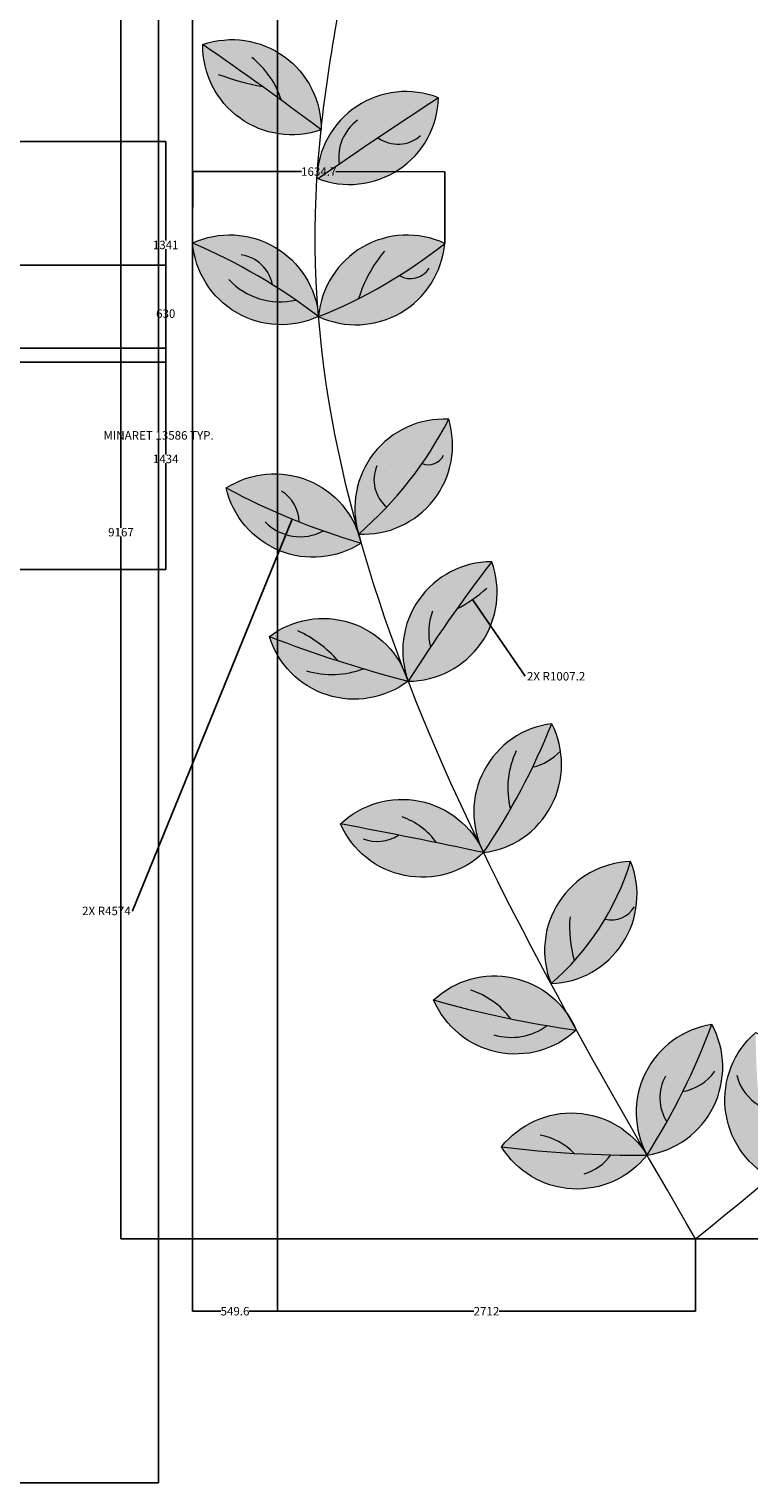
# Model space of a CAD drawing. Units: millimetres. Extents: x 8570 to 49085, y 3782 to 24863.
# Tile 12 of 15: x 35169 to 39837, y 5902 to 15329. Entities that reach past the tile are written whole.
import ezdxf

# ---------------------------------------------------------------- set-up
doc = ezdxf.new("R2010")
doc.units = ezdxf.units.MM
doc.header["$MEASUREMENT"] = 0
doc.header["$PDMODE"] = 3
for name, color, linetype, lineweight in [('A-ANNO-DIMS', 2, 'Continuous', 18), ('A-DETL-FOLI', 7, 'Continuous', 13), ('A-DETL-PATT', 3, 'Continuous', 13), ('A-DETL-STEM', 28, 'Continuous', 18)]:
    doc.layers.add(name, color=color, linetype=linetype, lineweight=lineweight)
doc.styles.get("Standard").update_dxf_attribs({"font": 'arial.ttf'})
doc.dimstyles.get("Standard").update_dxf_attribs({"dimtxt": 55, "dimasz": 0.18, "dimexe": 0.18, "dimexo": 0.0625, "dimgap": 0.09, "dimtad": 0, "dimtih": 1, "dimtoh": 1, "dimdec": 0, "dimzin": 0, "dimdsep": 46, "dimtxsty": 'Standard', "dimcen": 0.09, "dimadec": 0, "dimazin": 0, "dimtfac": 1, "dimtdec": 0, "dimtofl": 0, "dimtmove": 0, "dimatfit": 3, "dimfxl": 1, "dimtolj": 1, "dimtzin": 0, "dimarcsym": 0})

# ---------------------------------------------------------------- blocks, each defined once
blk = doc.blocks.new('*D15')
at = {"layer": 'A-ANNO-DIMS', "color": 0, "lineweight": -2, "transparency": 16777216}
for p, q in [((33971.1, 19487.3), (36009.1, 19487.3)), ((36008.9, 19487.1), (36008.9, 12722.6)), ((36008.9, 5901.7), (36008.9, 12666.2)), ((33971.1, 5901.5), (36009.1, 5901.5))]:
    blk.add_line(p, q, dxfattribs=at)
at = {"layer": 'A-ANNO-DIMS', "color": 0, "transparency": 16777216}
for points in [[(36008.8, 19487.1), (36008.9, 19487.1), (36008.9, 19487.3)], [(36008.8, 5901.7), (36008.9, 5901.7), (36008.9, 5901.5)]]:
    blk.add_solid(points, dxfattribs=at)
at = {"layer": 'Defpoints', "color": 0, "transparency": 16777216}
for p in [(33971, 19487.3), (36008.9, 19487.3), (33971, 5901.5)]:
    blk.add_point(p, dxfattribs=at)
at = {"layer": 'A-ANNO-DIMS', "color": 0, "transparency": 16777216, "insert": (36008.9, 12694.4), "char_height": 55, "attachment_point": 5}
blk.add_mtext('\\A1;MINARET 13586 TYP.', dxfattribs=at)
blk = doc.blocks.new('*D50')
at = {"layer": 'A-ANNO-DIMS', "color": 0, "lineweight": -2, "transparency": 16777216}
for p, q in [((22407.6, 13259), (36055.2, 13259)), ((36055, 13258.8), (36055, 12570.2)), ((36055, 11825.2), (36055, 12513.8)), ((24254.1, 11825), (36055.2, 11825))]:
    blk.add_line(p, q, dxfattribs=at)
at = {"layer": 'A-ANNO-DIMS', "color": 0, "transparency": 16777216}
for points in [[(36055, 13258.8), (36055, 13258.8), (36055, 13259)], [(36055, 11825.2), (36055, 11825.2), (36055, 11825)]]:
    blk.add_solid(points, dxfattribs=at)
at = {"layer": 'Defpoints', "color": 0, "transparency": 16777216}
for p in [(22407.5, 13259), (36055, 13259), (24254, 11825)]:
    blk.add_point(p, dxfattribs=at)
at = {"layer": 'A-ANNO-DIMS', "color": 0, "transparency": 16777216, "insert": (36055, 12542), "char_height": 55, "attachment_point": 5}
blk.add_mtext('\\A1;1434', dxfattribs=at)
blk = doc.blocks.new('*D51')
at = {"layer": 'A-ANNO-DIMS', "color": 0, "lineweight": -2, "transparency": 16777216}
for p, q in [((25004.1, 14600), (36055.2, 14600)), ((36055, 14599.8), (36055, 13957.7)), ((36055, 13259.2), (36055, 13901.3)), ((22407.6, 13259), (36055.2, 13259))]:
    blk.add_line(p, q, dxfattribs=at)
at = {"layer": 'A-ANNO-DIMS', "color": 0, "transparency": 16777216}
for points in [[(36055, 14599.8), (36055, 14599.8), (36055, 14600)], [(36055, 13259.2), (36055, 13259.2), (36055, 13259)]]:
    blk.add_solid(points, dxfattribs=at)
at = {"layer": 'Defpoints', "color": 0, "transparency": 16777216}
for p in [(25004, 14600), (36055, 14600), (22407.5, 13259)]:
    blk.add_point(p, dxfattribs=at)
at = {"layer": 'A-ANNO-DIMS', "color": 0, "transparency": 16777216, "insert": (36055, 13929.5), "char_height": 55, "attachment_point": 5}
blk.add_mtext('\\A1;1341', dxfattribs=at)
blk = doc.blocks.new('*D68')
at = {"layer": 'A-ANNO-DIMS', "color": 0, "lineweight": -2, "transparency": 16777216}
for p, q in [((29204.1, 13799), (36055.2, 13799)), ((36055, 13798.8), (36055, 13512.2)), ((36055, 13169.2), (36055, 13455.8)), ((28954.1, 13169), (36055.2, 13169))]:
    blk.add_line(p, q, dxfattribs=at)
at = {"layer": 'A-ANNO-DIMS', "color": 0, "transparency": 16777216}
for points in [[(36055, 13798.8), (36055, 13798.8), (36055, 13799)], [(36055, 13169.2), (36055, 13169.2), (36055, 13169)]]:
    blk.add_solid(points, dxfattribs=at)
at = {"layer": 'Defpoints', "color": 0, "transparency": 16777216}
for p in [(29204, 13799), (36055, 13799), (28954, 13169)]:
    blk.add_point(p, dxfattribs=at)
at = {"layer": 'A-ANNO-DIMS', "color": 0, "transparency": 16777216, "insert": (36055, 13484), "char_height": 55, "attachment_point": 5}
blk.add_mtext('\\A1;630', dxfattribs=at)
blk = doc.blocks.new('*D72')
at = {"layer": 'A-ANNO-DIMS', "color": 0, "lineweight": -2, "transparency": 16777216}
for p, q in [((36229.4, 13941.8), (36229.4, 17114.8)), ((36229.6, 17114.6), (40660.1, 17114.6)), ((45255, 17114.6), (40824.5, 17114.6)), ((45255.2, 15109.6), (45255.2, 17114.8))]:
    blk.add_line(p, q, dxfattribs=at)
at = {"layer": 'A-ANNO-DIMS', "color": 0, "transparency": 16777216}
for points in [[(36229.6, 17114.7), (36229.6, 17114.6), (36229.4, 17114.6)], [(45255, 17114.7), (45255, 17114.6), (45255.2, 17114.6)]]:
    blk.add_solid(points, dxfattribs=at)
at = {"layer": 'Defpoints', "color": 0, "transparency": 16777216}
for p in [(45255.2, 17114.6), (45255.2, 15109.5), (36229.4, 13941.8)]:
    blk.add_point(p, dxfattribs=at)
at = {"layer": 'A-ANNO-DIMS', "color": 0, "transparency": 16777216, "insert": (40742.3, 17114.6), "char_height": 55, "attachment_point": 5}
blk.add_mtext('\\A1;9026', dxfattribs=at)
blk = doc.blocks.new('*D73')
at = {"layer": 'A-ANNO-DIMS', "color": 0, "lineweight": -2, "transparency": 16777216}
for p, q in [((36779, 16650.1), (35764.8, 16650.1)), ((35764.9, 16649.9), (35764.9, 12095)), ((35764.9, 7483.7), (35764.9, 12038.6)), ((39490.9, 7483.5), (35764.8, 7483.5))]:
    blk.add_line(p, q, dxfattribs=at)
at = {"layer": 'A-ANNO-DIMS', "color": 0, "transparency": 16777216}
for points in [[(35764.9, 16649.9), (35765, 16649.9), (35764.9, 16650.1)], [(35764.9, 7483.7), (35765, 7483.7), (35764.9, 7483.5)]]:
    blk.add_solid(points, dxfattribs=at)
at = {"layer": 'Defpoints', "color": 0, "transparency": 16777216}
for p in [(35764.9, 16650.1), (36779.1, 16650.1), (39491, 7483.5)]:
    blk.add_point(p, dxfattribs=at)
at = {"layer": 'A-ANNO-DIMS', "color": 0, "transparency": 16777216, "insert": (35764.9, 12066.8), "char_height": 55, "attachment_point": 5}
blk.add_mtext('\\A1;9167', dxfattribs=at)
blk = doc.blocks.new('*D74')
at = {"layer": 'A-ANNO-DIMS', "color": 0, "lineweight": -2, "transparency": 16777216}
for p, q in [((36779.1, 16650.1), (36779.1, 7015)), ((36229.4, 13941.7), (36229.4, 7015)), ((36229.6, 7015.1), (36411.4, 7015.1)), ((36778.9, 7015.1), (36597.1, 7015.1))]:
    blk.add_line(p, q, dxfattribs=at)
at = {"layer": 'A-ANNO-DIMS', "color": 0, "transparency": 16777216}
for points in [[(36229.6, 7015.2), (36229.6, 7015.1), (36229.4, 7015.1)], [(36778.9, 7015.2), (36778.9, 7015.1), (36779.1, 7015.1)]]:
    blk.add_solid(points, dxfattribs=at)
at = {"layer": 'Defpoints', "color": 0, "transparency": 16777216}
for p in [(36779.1, 16650.1), (36229.4, 13941.8), (36779.1, 7015.1)]:
    blk.add_point(p, dxfattribs=at)
at = {"layer": 'A-ANNO-DIMS', "color": 0, "transparency": 16777216, "insert": (36504.3, 7015.1), "char_height": 55, "attachment_point": 5}
blk.add_mtext('\\A1;549.6', dxfattribs=at)
blk = doc.blocks.new('*D75')
at = {"layer": 'A-ANNO-DIMS', "color": 0, "lineweight": -2, "transparency": 16777216}
for p, q in [((36779.1, 16650.1), (36779.1, 7015)), ((39491, 7483.4), (39491, 7015)), ((36779.2, 7015.1), (38052.6, 7015.1)), ((39490.8, 7015.1), (38217.4, 7015.1))]:
    blk.add_line(p, q, dxfattribs=at)
at = {"layer": 'A-ANNO-DIMS', "color": 0, "transparency": 16777216}
for points in [[(36779.2, 7015.2), (36779.2, 7015.1), (36779.1, 7015.1)], [(39490.8, 7015.2), (39490.8, 7015.1), (39491, 7015.1)]]:
    blk.add_solid(points, dxfattribs=at)
at = {"layer": 'Defpoints', "color": 0, "transparency": 16777216}
for p in [(36779.1, 16650.1), (39491, 7483.5), (39491, 7015.1)]:
    blk.add_point(p, dxfattribs=at)
at = {"layer": 'A-ANNO-DIMS', "color": 0, "transparency": 16777216, "insert": (38135, 7015.1), "char_height": 55, "attachment_point": 5}
blk.add_mtext('\\A1;2712', dxfattribs=at)
blk = doc.blocks.new('*D76')
at = {"layer": 'A-ANNO-DIMS', "color": 0, "lineweight": -2, "transparency": 16777216}
for p, q in [((45255.3, 15109.5), (45721.9, 15109.5)), ((45721.7, 15109.3), (45721.7, 11324.7)), ((45721.7, 7483.7), (45721.7, 11268.3)), ((39491.1, 7483.5), (45721.9, 7483.5))]:
    blk.add_line(p, q, dxfattribs=at)
at = {"layer": 'A-ANNO-DIMS', "color": 0, "transparency": 16777216}
for points in [[(45721.6, 15109.3), (45721.7, 15109.3), (45721.7, 15109.5)], [(45721.6, 7483.7), (45721.7, 7483.7), (45721.7, 7483.5)]]:
    blk.add_solid(points, dxfattribs=at)
at = {"layer": 'Defpoints', "color": 0, "transparency": 16777216}
for p in [(45255.2, 15109.5), (45721.7, 15109.5), (39491, 7483.5)]:
    blk.add_point(p, dxfattribs=at)
at = {"layer": 'A-ANNO-DIMS', "color": 0, "transparency": 16777216, "insert": (45721.7, 11296.5), "char_height": 55, "attachment_point": 5}
blk.add_mtext('\\A1;7626', dxfattribs=at)
blk = doc.blocks.new('*D78')
at = {"layer": 'A-ANNO-DIMS', "color": 0, "lineweight": -2, "transparency": 16777216}
for p, q in [((36229.4, 13941.8), (36230, 14406.4)), ((36230.2, 14406.3), (36935.7, 14405.4)), ((37864.5, 14404.2), (37159, 14405.1)), ((37864.1, 13939.7), (37864.7, 14404.3))]:
    blk.add_line(p, q, dxfattribs=at)
at = {"layer": 'A-ANNO-DIMS', "color": 0, "transparency": 16777216}
for points in [[(36230.2, 14406.3), (36230.2, 14406.2), (36230, 14406.3)], [(37864.5, 14404.2), (37864.5, 14404.1), (37864.7, 14404.2)]]:
    blk.add_solid(points, dxfattribs=at)
at = {"layer": 'Defpoints', "color": 0, "transparency": 16777216}
for p in [(37864.7, 14404.2), (36229.4, 13941.8), (37864.1, 13939.7)]:
    blk.add_point(p, dxfattribs=at)
at = {"layer": 'A-ANNO-DIMS', "color": 0, "transparency": 16777216, "insert": (37047.4, 14405.2), "char_height": 55, "attachment_point": 5}
blk.add_mtext('\\A1;1634.7', dxfattribs=at)
blk = doc.blocks.new('*D95')
at = {"layer": 'A-ANNO-DIMS', "color": 0, "lineweight": -2, "transparency": 16777216}
for p, q in [((48826.8, 12322.2), (42401, 10673.8)), ((31690.9, 7926.2), (31691.1, 7926.2)), ((31691, 7926.2), (31691, 7926.3))]:
    blk.add_line(p, q, dxfattribs=at)
at = {"layer": 'A-ANNO-DIMS', "color": 0, "transparency": 16777216}
blk.add_solid([(42401, 10673.8), (42401, 10673.7), (42400.9, 10673.7)], dxfattribs=at)
at = {"layer": 'Defpoints', "color": 0, "transparency": 16777216}
for p in [(42400.9, 10673.7), (31691, 7926.2)]:
    blk.add_point(p, dxfattribs=at)
at = {"layer": 'A-ANNO-DIMS', "color": 0, "transparency": 16777216, "insert": (48956.7, 12322.2), "char_height": 55, "attachment_point": 5}
blk.add_mtext('\\A1;R11057', dxfattribs=at)
blk = doc.blocks.new('*D97')
at = {"layer": 'A-ANNO-DIMS', "color": 0, "lineweight": -2, "transparency": 16777216}
for p, q in [((38605.2, 16386.9), (38605.4, 16386.9)), ((38605.3, 16386.8), (38605.3, 16387)), ((35838.6, 9611), (36876, 12151.8)), ((35838.4, 9611), (35838.6, 9611))]:
    blk.add_line(p, q, dxfattribs=at)
at = {"layer": 'A-ANNO-DIMS', "color": 0, "transparency": 16777216}
blk.add_solid([(36876, 12151.8), (36876.1, 12151.8), (36876.1, 12152)], dxfattribs=at)
at = {"layer": 'Defpoints', "color": 0, "transparency": 16777216}
for p in [(38605.3, 16386.9), (36876.1, 12152)]:
    blk.add_point(p, dxfattribs=at)
at = {"layer": 'A-ANNO-DIMS', "color": 0, "transparency": 16777216, "insert": (35670.4, 9611), "char_height": 55, "attachment_point": 5}
blk.add_mtext('\\A1;2X R4574', dxfattribs=at)
blk = doc.blocks.new('*D99')
at = {"layer": 'A-ANNO-DIMS', "color": 0, "lineweight": -2, "transparency": 16777216}
for p, q in [((37473.5, 12460.3), (37473.6, 12460.3)), ((37473.6, 12460.2), (37473.6, 12460.4)), ((38386.6, 11132.5), (38044.3, 11630.3)), ((38386.8, 11132.5), (38386.6, 11132.5))]:
    blk.add_line(p, q, dxfattribs=at)
at = {"layer": 'A-ANNO-DIMS', "color": 0, "transparency": 16777216}
blk.add_solid([(38044.3, 11630.3), (38044.3, 11630.2), (38044.2, 11630.4)], dxfattribs=at)
at = {"layer": 'Defpoints', "color": 0, "transparency": 16777216}
for p in [(37473.6, 12460.3), (38044.2, 11630.4)]:
    blk.add_point(p, dxfattribs=at)
at = {"layer": 'A-ANNO-DIMS', "color": 0, "transparency": 16777216, "insert": (38586.6, 11132.5), "char_height": 55, "attachment_point": 5}
blk.add_mtext('\\A1;2X R1007.2', dxfattribs=at)

msp = doc.modelspace()

# ---------------------------------------------------------------- hatches: boundary and pattern name
at = {"layer": 'A-DETL-PATT'}
h = msp.add_hatch(color=256, dxfattribs=at)
h.dxf.hatch_style = 1
h.paths.add_polyline_path([(36295.31, 15228.7, 0.5205671), (37062.67, 14676.08, 0.0103411)])
h = msp.add_hatch(color=256, dxfattribs=at)
h.dxf.hatch_style = 1
h.paths.add_polyline_path([(36295.31, 15228.7, -0.0103411), (37062.67, 14676.08, 0.5205671)])
h = msp.add_hatch(color=256, dxfattribs=at)
h.dxf.hatch_style = 1
h.paths.add_polyline_path([(37823.87, 14883.96, 0.5205671), (37035.68, 14361.49, 0.0037395), (37043.74, 14358.39, -0.0070598)])
h = msp.add_hatch(color=256, dxfattribs=at)
h.dxf.hatch_style = 1
h.paths.add_polyline_path([(37823.87, 14883.96, 0.0070598), (37043.74, 14358.39, 0.5158234)])
h = msp.add_hatch(color=256, dxfattribs=at)
h.dxf.hatch_style = 1
h.paths.add_polyline_path([(36229.45, 13941.76, -0.520567), (37046.17, 13465.11, -0.520567), (37864.11, 13939.66, -0.520567), (37046.17, 13465.11, -0.520567)])
h = msp.add_hatch(color=256, dxfattribs=at)
h.dxf.hatch_style = 1
h.paths.add_polyline_path([(36229.45, 13941.76, -0.0616433), (37046.17, 13465.11, 0.5205671)])
h = msp.add_hatch(color=256, dxfattribs=at)
h.dxf.hatch_style = 1
h.paths.add_polyline_path([(37864.11, 13939.66, 0.5205671), (37046.17, 13465.11, 0.0744626)], flags=17)
h = msp.add_hatch(color=256, dxfattribs=at)
h.dxf.hatch_style = 1
h.paths.add_polyline_path([(36229.45, 13941.76, 0.520567), (37046.17, 13465.11, 0.0616433)], flags=17)
h = msp.add_hatch(color=256, dxfattribs=at)
h.dxf.hatch_style = 1
edge = h.paths.add_edge_path()
edge.add_arc((37858.74, 12222.44), 577.2, 86.889324, 194.195037)
edge.add_spline(control_points=[(37299.16, 12080.9), (37301.57, 12072.18), (37304, 12063.46), (37306.43, 12054.75)], knot_values=[4911.3561457, 4911.3561457, 4911.3561457, 4911.3561457, 4938.9064516, 4938.9064516, 4938.9064516, 4938.9064516], degree=3, periodic=0)
edge.add_arc((35669.24, 13939.89), 2496.83, 310.973454, 332.805194)
h = msp.add_hatch(color=256, dxfattribs=at)
h.dxf.hatch_style = 1
h.paths.add_polyline_path([(37890.06, 12798.79, -0.0955481), (37306.43, 12054.75, 0.5205671)])
h = msp.add_hatch(color=256, dxfattribs=at)
h.dxf.hatch_style = 1
h.paths.add_polyline_path([(36447.63, 12353.41, 0.0518202), (37323.1, 11995.94, 0.520567)])
h = msp.add_hatch(color=256, dxfattribs=at)
h.dxf.hatch_style = 1
h.paths.add_polyline_path([(36447.63, 12353.41, 0.5205671), (37323.1, 11995.94, -0.0518202)])
h = msp.add_hatch(color=256, dxfattribs=at)
h.dxf.hatch_style = 1
h.paths.add_polyline_path([(38169.31, 11875.19, 0.5048203), (37617.86, 11127.77, -0.0124698), (37627.03, 11100.49, -0.0213914)])
h = msp.add_hatch(color=256, dxfattribs=at)
h.dxf.hatch_style = 1
h.paths.add_polyline_path([(38169.31, 11875.19, 0.0213914), (37627.03, 11100.49, 0.5205671)])
h = msp.add_hatch(color=256, dxfattribs=at)
h.dxf.hatch_style = 1
h.paths.add_polyline_path([(36726.91, 11390.34, 0.0289339), (37627.03, 11100.49, -0.0124698), (37617.86, 11127.77, 0.5048203)])
h = msp.add_hatch(color=256, dxfattribs=at)
h.dxf.hatch_style = 1
h.paths.add_polyline_path([(37627.03, 11100.49, -0.0289339), (36726.91, 11390.34, 0.5205671)])
h = msp.add_hatch(color=256, dxfattribs=at)
h.dxf.hatch_style = 1
h.paths.add_polyline_path([(38558.32, 10824.89, 0.5013788), (38101.47, 10020.52, -0.0152167), (38116.54, 9988.79, 0.0525775)])
h = msp.add_hatch(color=256, dxfattribs=at)
h.dxf.hatch_style = 1
h.paths.add_polyline_path([(38558.32, 10824.89, -0.0171383), (38433.65, 10542.15, 0.1348282), (38615.59, 10646.7, 0.0816048)])
h = msp.add_hatch(color=256, dxfattribs=at)
h.dxf.hatch_style = 1
h.paths.add_polyline_path([(38615.59, 10646.7, -0.1348282), (38433.65, 10542.15, -0.0354074), (38116.54, 9988.79, 0.4210746)])
h = msp.add_hatch(color=256, dxfattribs=at)
h.dxf.hatch_style = 1
h.paths.add_polyline_path([(37189.36, 10174.71, -0.0070162), (38116.54, 9988.79, -0.0152167), (38101.47, 10020.52, 0.5013788)])
h = msp.add_hatch(color=256, dxfattribs=at)
h.dxf.hatch_style = 1
h.paths.add_polyline_path([(37189.36, 10174.71, 0.5205671), (38116.54, 9988.79, 0.0070162)])
h = msp.add_hatch(color=256, dxfattribs=at)
h.dxf.hatch_style = 1
h.paths.add_polyline_path([(39069.9, 9931.39, 0.520567), (38553.65, 9139.1, 0.1409243)])
h = msp.add_hatch(color=256, dxfattribs=at)
h.dxf.hatch_style = 1
h.paths.add_polyline_path([(39069.9, 9931.39, -0.1409243), (38553.65, 9139.1, 0.5205671)])
h = msp.add_hatch(color=256, dxfattribs=at)
h.dxf.hatch_style = 1
edge = h.paths.add_edge_path()
edge.add_spline(control_points=[(38717.84, 8838.28), (38699.24, 8871.96), (38680.7, 8905.65), (38662.23, 8939.34)], knot_values=[1468.6434181, 1468.6434181, 1468.6434181, 1468.6434181, 1577.9808208, 1577.9808208, 1577.9808208, 1577.9808208], degree=3, periodic=0)
edge.add_arc((38186.86, 8611.95), 577.2, 34.555708, 133.086732)
edge.add_arc((39646, 15528.1), 6753.9, 254.072359, 262.101105)
h = msp.add_hatch(color=256, dxfattribs=at)
h.dxf.hatch_style = 1
h.paths.add_polyline_path([(37792.57, 9033.49, 0.5205671), (38717.84, 8838.28, -0.0350464)])
h = msp.add_hatch(color=256, dxfattribs=at)
h.dxf.hatch_style = 1
h.paths.add_polyline_path([(39596.97, 8874.13, 0.520567), (39176.6, 8027.06, 0.0505737)])
h = msp.add_hatch(color=256, dxfattribs=at)
h.dxf.hatch_style = 1
h.paths.add_polyline_path([(39596.97, 8874.13, -0.0505737), (39176.6, 8027.06, 0.5205671)])
h = msp.add_hatch(color=256, dxfattribs=at)
h.dxf.hatch_style = 1
h.paths.add_polyline_path([(39881.17, 8822.47, 0.5205671), (39976.57, 7881.66, -0.0505737)])
h = msp.add_hatch(color=256, dxfattribs=at)
h.dxf.hatch_style = 1
h.paths.add_polyline_path([(38232.5, 8081.06, 0.0328597), (39176.6, 8027.06, 0.5205671)])
h = msp.add_hatch(color=256, dxfattribs=at)
h.dxf.hatch_style = 1
h.paths.add_polyline_path([(38232.5, 8081.06, 0.520567), (39176.6, 8027.06, -0.0328597)])

# ---------------------------------------------------------------- linework, layer by layer
at = {"layer": 'A-DETL-FOLI'}
for points in [[(37062.67, 14676.08, -0.520567), (36295.31, 15228.7, -0.520567)], [(37035.68, 14361.49, 0.5205671), (37823.87, 14883.96, 0.5205671)], [(37046.17, 13465.11, -0.5205671), (36229.45, 13941.76, -0.5205671)], [(37046.17, 13465.11, 0.5205671), (37864.11, 13939.66, 0.5205671)], [(37306.43, 12054.75, 0.5205671), (37890.06, 12798.79, 0.5205671)], [(37323.1, 11995.94, -0.5205671), (36447.63, 12353.41, -0.5205671)], [(37627.03, 11100.49, 0.5205671), (38169.31, 11875.19, 0.5205671)], [(37627.03, 11100.49, -0.5205671), (36726.91, 11390.34, -0.5205671)], [(38116.54, 9988.79, 0.5205671), (38558.32, 10824.89, 0.5205671)], [(38116.54, 9988.79, -0.5205671), (37189.36, 10174.71, -0.5205671)], [(38553.65, 9139.1, 0.5205671), (39069.9, 9931.39, 0.5205671)], [(38717.84, 8838.28, -0.5205671), (37792.57, 9033.49, -0.5205671)], [(39176.6, 8027.06, 0.5205671), (39596.97, 8874.13, 0.5205671)], [(39976.57, 7881.66, -0.5205671), (39881.17, 8822.47, -0.5205671)], [(39176.6, 8027.06, -0.5205671), (38232.5, 8081.06, -0.5205671)]]:
    msp.add_lwpolyline(points, format="xyb", close=True, dxfattribs=at)
for centre, radius, start, end in [((23320.55, -3596.85), 22863.63, 53.055085, 55.425), ((36271.19, 14703.58), 558.08, 17.051895, 52.17229), ((37032.61, 16773.69), 1850.87, 249.886877, 259.075602), ((56044.44, -13003.46), 33312.13, 123.15906, 124.777015), ((37476.65, 14496.91), 299.94, 126.268669, 188.510463), ((37560.28, 14802.57), 219.96, 234.307882, 311.816375), ((34712.07, 10403.74), 3849.69, 52.676825, 66.786584), ((36509.64, 13624.91), 242.64, 10.975798, 81.833743), ((35870.73, 16433.32), 3192.47, 291.604155, 308.638293), ((38138.63, 13327.54), 870.37, 139.909154, 163.015855), ((37643.87, 13851.05), 139.85, 238.748189, 328.478767), ((36798.02, 14020.4), 460, 223.326558, 282.722995), ((35669.24, 13939.89), 2496.83, 310.973454, 332.805194), ((37757.22, 12612.81), 108.88, 248.41912, 334.400323), ((37634.06, 12406.03), 228.57, 156.595932, 230.447825), ((38605.31, 16386.92), 4574.36, 241.855973, 253.721673), ((36680, 12126.54), 240.93, 1.777734, 58.42246), ((36927.75, 12356.22), 318.74, 224.316548, 298.113447), ((46947.91, 5153.12), 11056.67, 142.557509, 147.459302), ((37473.56, 12460.31), 1007.16, 297.810827, 311.215558), ((38161.62, 11414.85), 401.41, 159.701903, 193.541189), ((36563.49, 10690.41), 815.46, 41.653998, 64.77332), ((39679.3, 19016.27), 8177.5, 248.836039, 255.465354), ((37132.6, 11733.77), 589.63, 253.685845, 290.393138), ((34372.89, 12501.66), 4508.82, 326.129117, 338.167916), ((38838.71, 10406.9), 565.03, 154.67912, 194.042291), ((38334.29, 10925.66), 396.17, 284.524319, 315.239446), ((37434.91, 9784.63), 462.08, 35.512434, 70.735424), ((31028.6, -22953.94), 33696.62, 77.857396, 79.465354), ((37425.74, 10310.28), 249.31, 248.564819, 303.69009), ((37434.17, 10432.88), 1710.88, 310.86914, 342.95532), ((38947.21, 9723.28), 170.45, 255.51577, 329.955221), ((39431.86, 9504.6), 758.17, 174.789648, 196.615742), ((37864.29, 8585.96), 538.45, 37.132204, 71.607072), ((39646, 15528.1), 6753.9, 254.072359, 262.101105), ((38297.06, 9180.64), 390.09, 252.908213, 306.526234), ((35210.23, 10523.3), 4686.5, 327.815771, 339.396549), ((39546.84, 8398.85), 287.73, 150.652053, 212.713005), ((39357.43, 8748.48), 312.66, 279.345292, 325.49765), ((40061.17, 8620.56), 312.66, 193.8989, 240.051258), ((38402.78, 7743.64), 421.31, 44.425388, 79.130728), ((39114.91, 15229.08), 7202.28, 262.962572, 270.490744), ((38675.82, 8218.4), 326.41, 286.427156, 324.507445)]:
    msp.add_arc(centre, radius, start, end, dxfattribs=at)
at = {"layer": 'A-DETL-STEM'}
for points in [[(39491, 7483.5), (38190.27, 9726.55), (36625.55, 12424.85), (37154.41, 15335.42), (37243.63, 15826.48)], [(39491, 7483.5), (41497.86, 9125.36), (43912.02, 11100.44), (44441.22, 14010.96), (44530.5, 14502)]]:
    msp.add_open_spline(points, degree=3, knots=[0, 0, 0, 0, 7301.1442939, 8782.9420196, 8782.9420196, 8782.9420196, 8782.9420196], dxfattribs=at)

# ---------------------------------------------------------------- dimensions: what is measured, and where the dimension line sits
at = {"layer": 'A-ANNO-DIMS'}
dim = msp.add_linear_dim(base=(36008.87, 19487.32), p1=(33971, 5901.5), p2=(33971, 19487.32), angle=90, text='MINARET <> TYP.', dimstyle='Standard', override={"dimdec": 0, "dimlfac": 1, "dimrnd": 0, "dimzin": 0, "dimdsep": 46, "dimlunit": 2}, dxfattribs=at)
dim.commit()
dim.dimension.update_dxf_attribs({"geometry": '*D15', "text_midpoint": (36008.87, 12694.41)})
for base, p1, p2, override, picture, middle in [((45255.2, 17114.63), (36229.45, 13941.76), (45255.2, 15109.49), {"dimdec": 0, "dimlfac": 1, "dimrnd": 0, "dimzin": 0, "dimdsep": 46, "dimlunit": 2}, '*D72', (40742.32, 17114.63)), ((36779.06, 7015.15), (36229.45, 13941.76), (36779.06, 16650.13), {"dimdec": 1, "dimlfac": 1, "dimrnd": 0, "dimzin": 0, "dimdsep": 46, "dimlunit": 2}, '*D74', (36504.25, 7015.15)), ((39491, 7015.15), (36779.06, 16650.13), (39491, 7483.5), {"dimdec": 0, "dimlfac": 1, "dimrnd": 0, "dimzin": 0, "dimdsep": 46, "dimlunit": 2}, '*D75', (38135.03, 7015.15))]:
    dim = msp.add_linear_dim(base=base, p1=p1, p2=p2, dimstyle='Standard', override=override, dxfattribs=at)
    dim.commit()
    dim.dimension.update_dxf_attribs({"geometry": picture, "text_midpoint": middle})
for base, p1, p2, angle, override, picture, middle in [((35764.95, 16650.13), (39491, 7483.5), (36779.06, 16650.13), 90, {"dimdec": 0, "dimlfac": 1, "dimrnd": 0, "dimzin": 0, "dimdsep": 46, "dimlunit": 2}, '*D73', (35764.95, 12066.81)), ((45721.68, 15109.49), (39491, 7483.5), (45255.2, 15109.49), 90, {"dimdec": 0, "dimlfac": 1, "dimrnd": 0, "dimzin": 0, "dimdsep": 46, "dimlunit": 2}, '*D76', (45721.68, 11296.49)), ((36055, 14600), (22407.5, 13259), (25004, 14600), 90, {"dimdec": 0, "dimlfac": 1, "dimrnd": 0, "dimzin": 0, "dimdsep": 46, "dimlunit": 2}, '*D51', (36055, 13929.5)), ((37864.71, 14404.16), (36229.45, 13941.76), (37864.11, 13939.66), 359.926464, {"dimdec": 1, "dimlfac": 1, "dimrnd": 0, "dimzin": 0, "dimdsep": 46, "dimlunit": 2}, '*D78', (37047.38, 14405.21)), ((36055, 13799), (28954, 13169), (29204, 13799), 90, {"dimdec": 0, "dimlfac": 1, "dimrnd": 0, "dimzin": 0, "dimdsep": 46, "dimlunit": 2}, '*D68', (36055, 13484)), ((36055, 13259), (24254, 11825), (22407.5, 13259), 90, {"dimdec": 0, "dimlfac": 1, "dimrnd": 0, "dimzin": 0, "dimdsep": 46, "dimlunit": 2}, '*D50', (36055, 12542))]:
    dim = msp.add_linear_dim(base=base, p1=p1, p2=p2, angle=angle, dimstyle='Standard', override=override, dxfattribs=at)
    dim.commit()
    dim.dimension.update_dxf_attribs({"geometry": picture, "text_midpoint": middle})
for center, mpoint, override, picture, middle in [((38605.31, 16386.92), (36876.1, 12151.99), {"dimdec": 0, "dimlfac": 1, "dimrnd": 0, "dimzin": 0, "dimdsep": 46, "dimlunit": 2}, '*D97', (35670.42, 9611.04)), ((37473.56, 12460.31), (38044.21, 11630.41), {"dimdec": 1, "dimlfac": 1, "dimrnd": 0, "dimzin": 0, "dimdsep": 46, "dimlunit": 2}, '*D99', (38586.63, 11132.47))]:
    dim = msp.add_radius_dim(center=center, mpoint=mpoint, text='2X <>', dimstyle='Standard', override=override, dxfattribs=at)
    dim.commit()
    dim.dimension.update_dxf_attribs({"geometry": picture, "text_midpoint": middle, "dimtype": 164})
dim = msp.add_radius_dim(center=(31690.99, 7926.25), mpoint=(42400.86, 10673.71), dimstyle='Standard', override={"dimdec": 0, "dimlfac": 1, "dimrnd": 0, "dimzin": 0, "dimdsep": 46, "dimlunit": 2}, dxfattribs=at)
dim.commit()
dim.dimension.update_dxf_attribs({"geometry": '*D95', "text_midpoint": (48826.79, 12322.19), "dimtype": 164})

doc.saveas('drawing.dxf')
